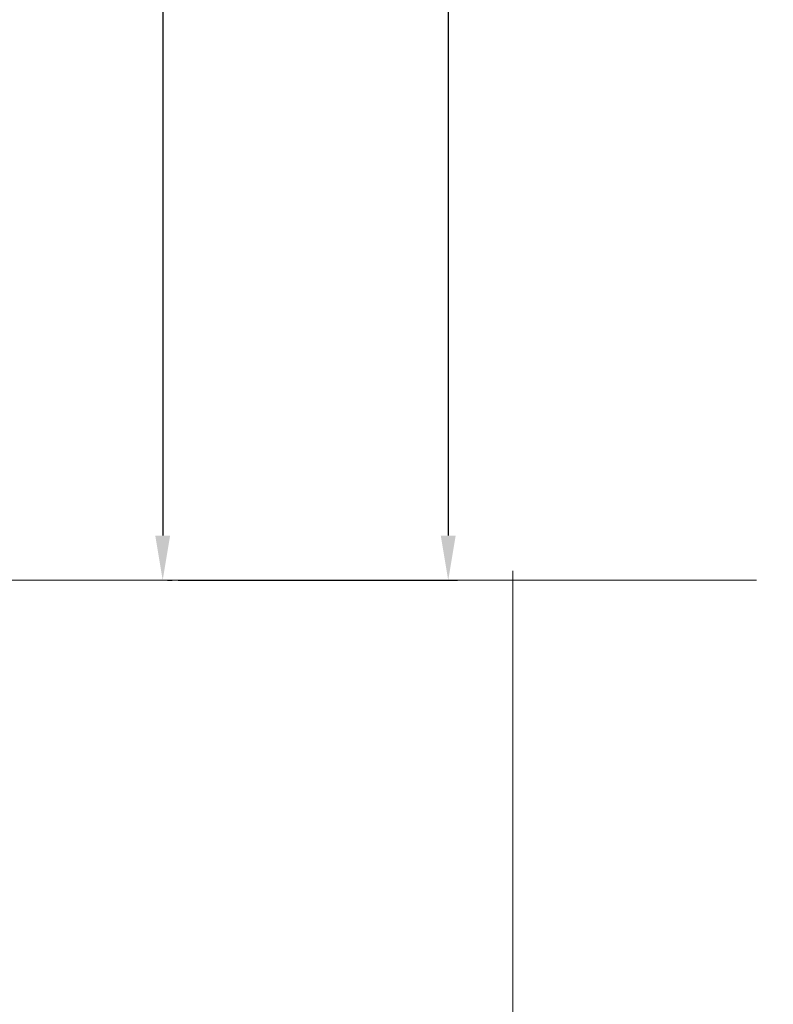
# Model space of a CAD drawing. Units: millimetres. Extents: x 595116 to 630915, y 909473 to 920225.
# Tile 110 of 134: x 629845 to 629946, y 919085 to 919217. Entities that reach past the tile are written whole.
import ezdxf

# ---------------------------------------------------------------- set-up
doc = ezdxf.new("R2010")
doc.units = ezdxf.units.MM
doc.layers.add('C-ROAD', color=30, linetype='Continuous', lineweight=18)
doc.layers.add('Dimension', color=3, linetype='Continuous', lineweight=18)
doc.styles.get("Standard").update_dxf_attribs({"font": 'arial.ttf'})
doc.dimstyles.new('ISO-25', dxfattribs={"dimtxt": 9, "dimasz": 6, "dimexe": 1.25, "dimexo": 0.625, "dimtad": 1, "dimlunit": 4, "dimtxsty": 'Standard', "dimcen": 2.5, "dimadec": 0, "dimazin": 0, "dimtfac": 1, "dimtmove": 0, "dimatfit": 3, "dimfxl": 1, "dimarcsym": 0})

# ---------------------------------------------------------------- blocks, each defined once
blk = doc.blocks.new('*D123')
at = {"layer": 'Defpoints', "color": 0, "transparency": 16777216}
for p in [(629864.28, 919369.93), (629864.28, 919141.93), (629864.28, 919141.93)]:
    blk.add_point(p, dxfattribs=at)
at = {"layer": 'Dimension', "color": 0, "lineweight": -2, "transparency": 16777216}
for p, q in [((629864.91, 919369.93), (629865.53, 919369.93)), ((629864.28, 919363.93), (629864.28, 919147.93)), ((629864.91, 919141.93), (629865.53, 919141.93))]:
    blk.add_line(p, q, dxfattribs=at)
at = {"layer": 'Dimension', "color": 0, "transparency": 16777216}
for points in [[(629863.28, 919363.93), (629865.28, 919363.93), (629864.28, 919369.93)], [(629863.28, 919147.93), (629865.28, 919147.93), (629864.28, 919141.93)]]:
    blk.add_solid(points, dxfattribs=at)
at = {"layer": 'Dimension', "color": 0, "transparency": 16777216, "insert": (629857.53, 919255.93), "char_height": 12, "attachment_point": 5, "rotation": 90}
blk.add_mtext("19'", dxfattribs=at)
blk = doc.blocks.new('*D124')
at = {"layer": 'Defpoints', "color": 0, "transparency": 16777216}
for p in [(629865.75, 920084.93), (629865.75, 919141.93), (629902.57, 919141.93)]:
    blk.add_point(p, dxfattribs=at)
at = {"layer": 'Dimension', "color": 0, "lineweight": -2, "transparency": 16777216}
for p, q in [((629866.37, 920084.93), (629903.82, 920084.93)), ((629902.57, 920078.93), (629902.57, 919147.93)), ((629866.37, 919141.93), (629903.82, 919141.93))]:
    blk.add_line(p, q, dxfattribs=at)
at = {"layer": 'Dimension', "color": 0, "transparency": 16777216}
for points in [[(629901.57, 920078.93), (629903.57, 920078.93), (629902.57, 920084.93)], [(629901.57, 919147.93), (629903.57, 919147.93), (629902.57, 919141.93)]]:
    blk.add_solid(points, dxfattribs=at)
at = {"layer": 'Dimension', "color": 0, "transparency": 16777216, "insert": (629897.35, 919613.43), "char_height": 9, "attachment_point": 5, "rotation": 90}
blk.add_mtext('78\'-7"', dxfattribs=at)

msp = doc.modelspace()

# ---------------------------------------------------------------- linework, layer by layer
at = {"layer": 'C-ROAD'}
msp.add_line((629842.541, 919141.928), (629943.895, 919141.928), dxfattribs=at)
msp.add_lwpolyline([(629911.25, 919143.178), (629911.25, 919062.342), (629946.162, 919021.992), (629869.502, 919021.872), (629911.25, 918997.995), (629911.25, 918900.678)], dxfattribs=at)

# ---------------------------------------------------------------- dimensions: what is measured, and where the dimension line sits
at = {"layer": 'Dimension'}
for base, p1, p2, override, picture, middle in [((629902.574, 919141.928), (629865.746, 920084.928), (629865.746, 919141.928), {"dimclrd": 0, "dimclre": 0, "dimclrt": 0}, '*D124', (629897.354, 919613.428)), ((629864.281, 919141.928), (629864.281, 919369.928), (629864.281, 919141.928), {"dimtxt": 12, "dimclrd": 0, "dimclre": 0, "dimclrt": 0}, '*D123', (629857.529, 919255.928))]:
    dim = msp.add_linear_dim(base=base, p1=p1, p2=p2, angle=90, dimstyle='ISO-25', override=override, dxfattribs=at)
    dim.commit()
    dim.dimension.update_dxf_attribs({"geometry": picture, "text_midpoint": middle})

doc.saveas('drawing.dxf')
